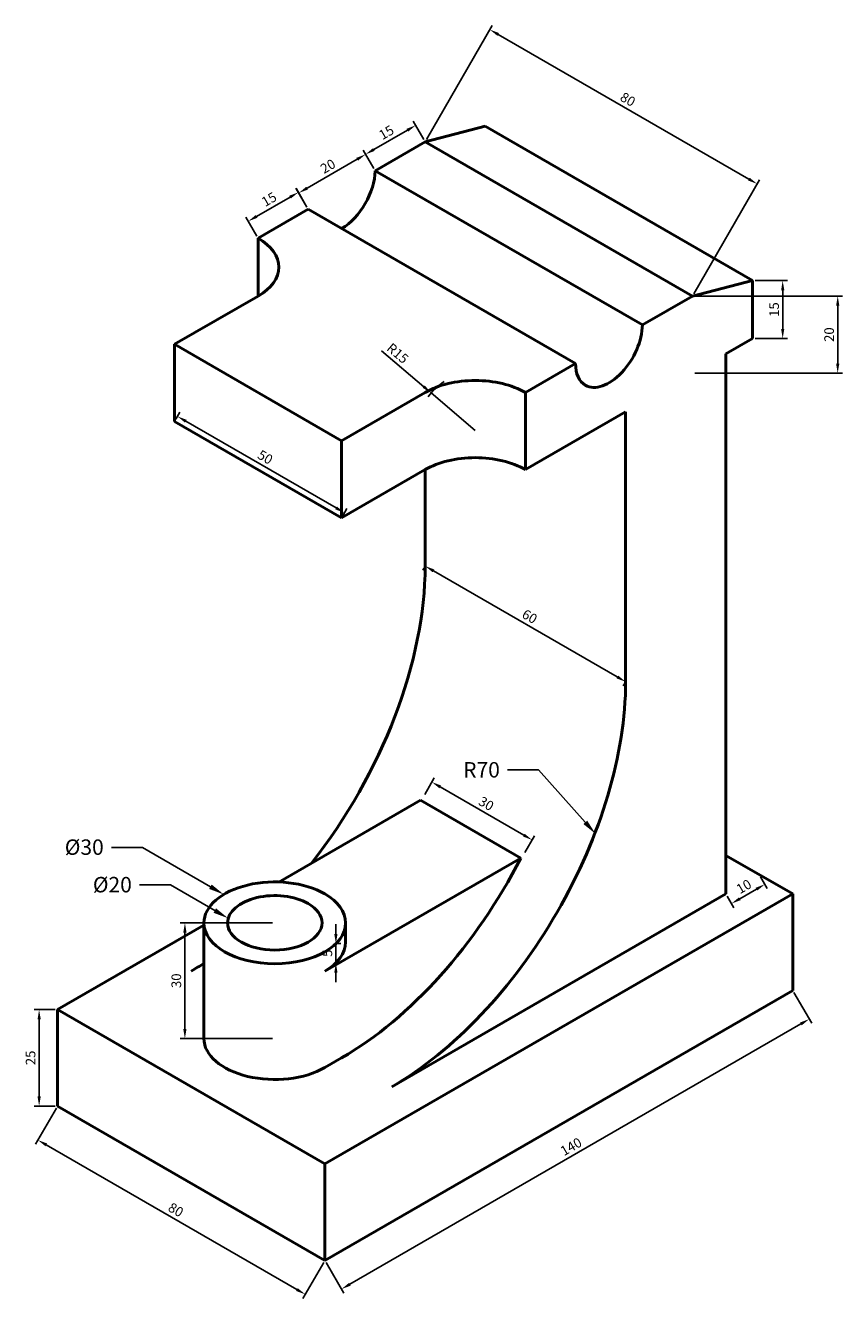
# Model space of a CAD drawing. Units: millimetres. Extents: x 2160 to 2371, y 1190 to 1520.
import ezdxf
from ezdxf import colors
from ezdxf.entities.mleader import LeaderData, LeaderLine
from ezdxf.math import Vec2, Vec3

# ---------------------------------------------------------------- set-up
doc = ezdxf.new("R2010")
doc.units = ezdxf.units.MM
for name, color, linetype, lineweight in [('M-DIMS', 2, 'Continuous', 25), ('M-OUTL', 7, 'Continuous', 50), ('M-TEXT', 3, 'Continuous', 25)]:
    doc.layers.add(name, color=color, linetype=linetype, lineweight=lineweight)
doc.styles.get("Standard").update_dxf_attribs({"font": 'arial.ttf'})
doc.dimstyles.new('ISO-25', dxfattribs={"dimtxt": 2.5, "dimasz": 2.5, "dimexe": 1.25, "dimexo": 0.625, "dimtad": 1, "dimtxsty": 'Standard', "dimcen": 2.5, "dimadec": 0, "dimazin": 0, "dimtfac": 1, "dimtmove": 0, "dimatfit": 3, "dimfxl": 1, "dimarcsym": 0})

# ---------------------------------------------------------------- blocks, each defined once
blk = doc.blocks.new('*D1')
at = {"layer": 'Defpoints', "color": 0, "transparency": 16777216}
for p in [(2167.87, 1239.87), (2237.16, 1199.87), (2232.07, 1191.06)]:
    blk.add_point(p, dxfattribs=at)
at = {"layer": 'M-DIMS', "color": 0, "lineweight": -2, "transparency": 16777216}
for p, q in [((2167.56, 1239.33), (2162.16, 1229.98)), ((2164.95, 1229.81), (2229.9, 1192.31)), ((2236.84, 1199.33), (2231.44, 1189.98))]:
    blk.add_line(p, q, dxfattribs=at)
at = {"layer": 'M-DIMS', "color": 0, "transparency": 16777216}
for points in [[(2165.16, 1230.17), (2164.74, 1229.45), (2162.79, 1231.06)], [(2230.11, 1192.67), (2229.69, 1191.95), (2232.07, 1191.06)]]:
    blk.add_solid(points, dxfattribs=at)
at = {"layer": 'M-DIMS', "color": 0, "transparency": 16777216, "insert": (2198.38, 1212.71), "char_height": 2.5, "attachment_point": 5, "rotation": 330}
blk.add_mtext('80', dxfattribs=at)
blk = doc.blocks.new('*D2')
at = {"layer": 'Defpoints', "color": 0, "transparency": 16777216}
for p in [(2358.4, 1269.87), (2362.7, 1262.43), (2237.16, 1199.87)]:
    blk.add_point(p, dxfattribs=at)
at = {"layer": 'M-DIMS', "color": 0, "lineweight": -2, "transparency": 16777216}
for p, q in [((2358.71, 1269.33), (2363.32, 1261.35)), ((2243.62, 1193.68), (2360.53, 1261.18)), ((2237.47, 1199.33), (2242.08, 1191.35))]:
    blk.add_line(p, q, dxfattribs=at)
at = {"layer": 'M-DIMS', "color": 0, "transparency": 16777216}
for points in [[(2360.32, 1261.54), (2360.74, 1260.82), (2362.7, 1262.43)], [(2243.41, 1194.04), (2243.83, 1193.32), (2241.45, 1192.43)]]:
    blk.add_solid(points, dxfattribs=at)
at = {"layer": 'M-DIMS', "color": 0, "transparency": 16777216, "insert": (2301.12, 1229.08), "char_height": 2.5, "attachment_point": 5, "rotation": 30}
blk.add_mtext('140', dxfattribs=at)
blk = doc.blocks.new('*D3')
at = {"layer": 'Defpoints', "color": 0, "transparency": 16777216}
for p in [(2224.16, 1287.37), (2200.87, 1257.37), (2224.16, 1257.37)]:
    blk.add_point(p, dxfattribs=at)
at = {"layer": 'M-DIMS', "color": 0, "lineweight": -2, "transparency": 16777216}
for p, q in [((2223.54, 1287.37), (2199.62, 1287.37)), ((2200.87, 1284.87), (2200.87, 1259.87)), ((2223.54, 1257.37), (2199.62, 1257.37))]:
    blk.add_line(p, q, dxfattribs=at)
at = {"layer": 'M-DIMS', "color": 0, "transparency": 16777216}
for points in [[(2200.45, 1284.87), (2201.29, 1284.87), (2200.87, 1287.37)], [(2200.45, 1259.87), (2201.29, 1259.87), (2200.87, 1257.37)]]:
    blk.add_solid(points, dxfattribs=at)
at = {"layer": 'M-DIMS', "color": 0, "transparency": 16777216, "insert": (2198.97, 1272.37), "char_height": 2.5, "attachment_point": 5, "rotation": 90}
blk.add_mtext('30', dxfattribs=at)
blk = doc.blocks.new('*D4')
at = {"layer": 'Defpoints', "color": 0, "transparency": 16777216}
for p in [(2240, 1282), (2240, 1277), (2240, 1277)]:
    blk.add_point(p, dxfattribs=at)
at = {"layer": 'M-DIMS', "color": 0, "lineweight": -2, "transparency": 16777216}
for p, q in [((2240, 1284.5), (2240, 1287)), ((2240, 1282), (2240, 1277)), ((2240.63, 1282), (2241.25, 1282)), ((2240, 1274.5), (2240, 1272)), ((2240.63, 1277), (2241.25, 1277))]:
    blk.add_line(p, q, dxfattribs=at)
at = {"layer": 'M-DIMS', "color": 0, "transparency": 16777216}
for points in [[(2239.59, 1284.5), (2240.42, 1284.5), (2240, 1282)], [(2239.59, 1274.5), (2240.42, 1274.5), (2240, 1277)]]:
    blk.add_solid(points, dxfattribs=at)
at = {"layer": 'M-DIMS', "color": 0, "transparency": 16777216, "insert": (2238.11, 1279.5), "char_height": 2.5, "attachment_point": 5, "rotation": 90}
blk.add_mtext('5', dxfattribs=at)
blk = doc.blocks.new('*D5')
at = {"layer": 'Defpoints', "color": 0, "transparency": 16777216}
for p in [(2167.87, 1264.87), (2163.09, 1239.87), (2167.87, 1239.87)]:
    blk.add_point(p, dxfattribs=at)
at = {"layer": 'M-DIMS', "color": 0, "lineweight": -2, "transparency": 16777216}
for p, q in [((2167.25, 1264.87), (2161.84, 1264.87)), ((2163.09, 1262.37), (2163.09, 1242.37)), ((2167.25, 1239.87), (2161.84, 1239.87))]:
    blk.add_line(p, q, dxfattribs=at)
at = {"layer": 'M-DIMS', "color": 0, "transparency": 16777216}
for points in [[(2162.68, 1262.37), (2163.51, 1262.37), (2163.09, 1264.87)], [(2162.68, 1242.37), (2163.51, 1242.37), (2163.09, 1239.87)]]:
    blk.add_solid(points, dxfattribs=at)
at = {"layer": 'M-DIMS', "color": 0, "transparency": 16777216, "insert": (2161.19, 1252.37), "char_height": 2.5, "attachment_point": 5, "rotation": 90}
blk.add_mtext('25', dxfattribs=at)
blk = doc.blocks.new('*D6')
at = {"layer": 'Defpoints', "color": 0, "transparency": 16777216}
for p in [(2262.71, 1320.11), (2290.86, 1308.87), (2288.69, 1305.11)]:
    blk.add_point(p, dxfattribs=at)
at = {"layer": 'M-DIMS', "color": 0, "lineweight": -2, "transparency": 16777216}
for p, q in [((2263.03, 1320.65), (2265.51, 1324.95)), ((2267.05, 1322.62), (2288.7, 1310.12)), ((2289.01, 1305.65), (2291.49, 1309.95))]:
    blk.add_line(p, q, dxfattribs=at)
at = {"layer": 'M-DIMS', "color": 0, "transparency": 16777216}
for points in [[(2267.26, 1322.98), (2266.84, 1322.26), (2264.88, 1323.87)], [(2288.91, 1310.48), (2288.49, 1309.76), (2290.86, 1308.87)]]:
    blk.add_solid(points, dxfattribs=at)
at = {"layer": 'M-DIMS', "color": 0, "transparency": 16777216, "insert": (2278.82, 1318.02), "char_height": 2.5, "attachment_point": 5, "rotation": 330}
blk.add_mtext('30', dxfattribs=at)
blk = doc.blocks.new('*D7')
at = {"layer": 'Defpoints', "color": 0, "transparency": 16777216}
for p in [(2263.14, 1379.87), (2315.1, 1349.87), (2315.1, 1349.87)]:
    blk.add_point(p, dxfattribs=at)
at = {"layer": 'M-DIMS', "color": 0, "lineweight": -2, "transparency": 16777216}
for p, q in [((2262.82, 1379.33), (2262.51, 1378.79)), ((2265.3, 1378.62), (2312.93, 1351.12)), ((2314.78, 1349.33), (2314.47, 1348.79))]:
    blk.add_line(p, q, dxfattribs=at)
at = {"layer": 'M-DIMS', "color": 0, "transparency": 16777216}
for points in [[(2265.51, 1378.99), (2265.09, 1378.26), (2263.14, 1379.87)], [(2313.14, 1351.49), (2312.72, 1350.76), (2315.1, 1349.87)]]:
    blk.add_solid(points, dxfattribs=at)
at = {"layer": 'M-DIMS', "color": 0, "transparency": 16777216, "insert": (2290.07, 1366.52), "char_height": 2.5, "attachment_point": 5, "rotation": 330}
blk.add_mtext('60', dxfattribs=at)
blk = doc.blocks.new('*D8')
at = {"layer": 'Defpoints', "color": 0, "transparency": 16777216}
for p in [(2279.92, 1518.94), (2263.14, 1489.87), (2332.42, 1449.87)]:
    blk.add_point(p, dxfattribs=at)
at = {"layer": 'M-DIMS', "color": 0, "lineweight": -2, "transparency": 16777216}
for p, q in [((2263.45, 1490.42), (2280.54, 1520.02)), ((2347.03, 1480.19), (2282.08, 1517.69)), ((2332.73, 1450.42), (2349.82, 1480.02))]:
    blk.add_line(p, q, dxfattribs=at)
at = {"layer": 'M-DIMS', "color": 0, "transparency": 16777216}
for points in [[(2282.29, 1518.05), (2281.87, 1517.33), (2279.92, 1518.94)], [(2347.24, 1480.55), (2346.83, 1479.83), (2349.2, 1478.94)]]:
    blk.add_solid(points, dxfattribs=at)
at = {"layer": 'M-DIMS', "color": 0, "transparency": 16777216, "insert": (2315.51, 1500.59), "char_height": 2.5, "attachment_point": 5, "rotation": 330}
blk.add_mtext('80', dxfattribs=at)
blk = doc.blocks.new('*D9')
at = {"layer": 'Defpoints', "color": 0, "transparency": 16777216}
for p in [(2348.01, 1453.87), (2348.01, 1438.87), (2355.8, 1438.87)]:
    blk.add_point(p, dxfattribs=at)
at = {"layer": 'M-DIMS', "color": 0, "lineweight": -2, "transparency": 16777216}
for p, q in [((2348.63, 1453.87), (2357.05, 1453.87)), ((2355.8, 1451.37), (2355.8, 1441.37)), ((2348.63, 1438.87), (2357.05, 1438.87))]:
    blk.add_line(p, q, dxfattribs=at)
at = {"layer": 'M-DIMS', "color": 0, "transparency": 16777216}
for points in [[(2355.39, 1451.37), (2356.22, 1451.37), (2355.8, 1453.87)], [(2355.39, 1441.37), (2356.22, 1441.37), (2355.8, 1438.87)]]:
    blk.add_solid(points, dxfattribs=at)
at = {"layer": 'M-DIMS', "color": 0, "transparency": 16777216, "insert": (2353.9, 1446.37), "char_height": 2.5, "attachment_point": 5, "rotation": 90}
blk.add_mtext('15', dxfattribs=at)
blk = doc.blocks.new('*D10')
at = {"layer": 'Defpoints', "color": 0, "transparency": 16777216}
for p in [(2263.14, 1489.87), (2247.7, 1486.62), (2250.15, 1482.37)]:
    blk.add_point(p, dxfattribs=at)
at = {"layer": 'M-DIMS', "color": 0, "lineweight": -2, "transparency": 16777216}
for p, q in [((2262.82, 1490.42), (2260.06, 1495.2)), ((2258.52, 1492.87), (2249.86, 1487.87)), ((2249.83, 1482.92), (2247.07, 1487.7))]:
    blk.add_line(p, q, dxfattribs=at)
at = {"layer": 'M-DIMS', "color": 0, "transparency": 16777216}
for points in [[(2258.31, 1493.23), (2258.73, 1492.5), (2260.69, 1494.12)], [(2249.65, 1488.23), (2250.07, 1487.5), (2247.7, 1486.62)]]:
    blk.add_solid(points, dxfattribs=at)
at = {"layer": 'M-DIMS', "color": 0, "transparency": 16777216, "insert": (2253.24, 1492.01), "char_height": 2.5, "attachment_point": 5, "rotation": 30}
blk.add_mtext('15', dxfattribs=at)
blk = doc.blocks.new('*D11')
at = {"layer": 'Defpoints', "color": 0, "transparency": 16777216}
for p in [(2230.29, 1476.77), (2232.83, 1472.37), (2219.83, 1464.87)]:
    blk.add_point(p, dxfattribs=at)
at = {"layer": 'M-DIMS', "color": 0, "lineweight": -2, "transparency": 16777216}
for p, q in [((2219.46, 1470.52), (2228.12, 1475.52)), ((2232.51, 1472.92), (2229.66, 1477.86)), ((2219.52, 1465.42), (2216.67, 1470.36))]:
    blk.add_line(p, q, dxfattribs=at)
at = {"layer": 'M-DIMS', "color": 0, "transparency": 16777216}
for points in [[(2227.91, 1475.88), (2228.33, 1475.16), (2230.29, 1476.77)], [(2219.25, 1470.88), (2219.67, 1470.16), (2217.3, 1469.27)]]:
    blk.add_solid(points, dxfattribs=at)
at = {"layer": 'M-DIMS', "color": 0, "transparency": 16777216, "insert": (2222.84, 1474.67), "char_height": 2.5, "attachment_point": 5, "rotation": 30}
blk.add_mtext('15', dxfattribs=at)
blk = doc.blocks.new('*D12')
at = {"layer": 'Defpoints', "color": 0, "transparency": 16777216}
for p in [(2247.71, 1486.6), (2250.15, 1482.37), (2232.83, 1472.37)]:
    blk.add_point(p, dxfattribs=at)
at = {"layer": 'M-DIMS', "color": 0, "lineweight": -2, "transparency": 16777216}
for p, q in [((2232.55, 1477.85), (2245.54, 1485.35)), ((2249.83, 1482.92), (2247.08, 1487.68)), ((2232.51, 1472.92), (2229.76, 1477.68))]:
    blk.add_line(p, q, dxfattribs=at)
at = {"layer": 'M-DIMS', "color": 0, "transparency": 16777216}
for points in [[(2245.33, 1485.71), (2245.75, 1484.99), (2247.71, 1486.6)], [(2232.34, 1478.21), (2232.76, 1477.49), (2230.39, 1476.6)]]:
    blk.add_solid(points, dxfattribs=at)
at = {"layer": 'M-DIMS', "color": 0, "transparency": 16777216, "insert": (2238.1, 1483.25), "char_height": 2.5, "attachment_point": 5, "rotation": 30}
blk.add_mtext('20', dxfattribs=at)
blk = doc.blocks.new('*D13')
at = {"layer": 'Defpoints', "color": 0, "transparency": 16777216}
for p in [(2198.18, 1417.37), (2198.94, 1418.68), (2241.49, 1392.37)]:
    blk.add_point(p, dxfattribs=at)
at = {"layer": 'M-DIMS', "color": 0, "lineweight": -2, "transparency": 16777216}
for p, q in [((2198.5, 1417.92), (2199.56, 1419.76)), ((2240.07, 1394.93), (2201.1, 1417.43)), ((2241.8, 1392.92), (2242.86, 1394.76))]:
    blk.add_line(p, q, dxfattribs=at)
at = {"layer": 'M-DIMS', "color": 0, "transparency": 16777216}
for points in [[(2201.31, 1417.79), (2200.89, 1417.07), (2198.94, 1418.68)], [(2240.28, 1395.29), (2239.87, 1394.57), (2242.24, 1393.68)]]:
    blk.add_solid(points, dxfattribs=at)
at = {"layer": 'M-DIMS', "color": 0, "transparency": 16777216, "insert": (2221.54, 1407.83), "char_height": 2.5, "attachment_point": 5, "rotation": 330}
blk.add_mtext('50', dxfattribs=at)
blk = doc.blocks.new('*D14')
at = {"layer": 'Defpoints', "color": 0, "transparency": 16777216}
for p in [(2332.42, 1449.87), (2332.42, 1429.87), (2370.06, 1429.87)]:
    blk.add_point(p, dxfattribs=at)
at = {"layer": 'M-DIMS', "color": 0, "lineweight": -2, "transparency": 16777216}
for p, q in [((2333.04, 1449.87), (2371.31, 1449.87)), ((2370.06, 1447.37), (2370.06, 1432.37)), ((2333.04, 1429.87), (2371.31, 1429.87))]:
    blk.add_line(p, q, dxfattribs=at)
at = {"layer": 'M-DIMS', "color": 0, "transparency": 16777216}
for points in [[(2369.64, 1447.37), (2370.48, 1447.37), (2370.06, 1449.87)], [(2369.64, 1432.37), (2370.48, 1432.37), (2370.06, 1429.87)]]:
    blk.add_solid(points, dxfattribs=at)
at = {"layer": 'M-DIMS', "color": 0, "transparency": 16777216, "insert": (2368.16, 1439.87), "char_height": 2.5, "attachment_point": 5, "rotation": 90}
blk.add_mtext('20', dxfattribs=at)
blk = doc.blocks.new('*D15')
at = {"layer": 'Defpoints', "color": 0, "transparency": 16777216}
for p in [(2349.74, 1299.87), (2351.18, 1297.37), (2341.08, 1294.87)]:
    blk.add_point(p, dxfattribs=at)
at = {"layer": 'M-DIMS', "color": 0, "lineweight": -2, "transparency": 16777216}
for p, q in [((2350.05, 1299.33), (2351.81, 1296.29)), ((2341.39, 1294.33), (2343.15, 1291.29)), ((2344.69, 1293.62), (2349.02, 1296.12))]:
    blk.add_line(p, q, dxfattribs=at)
at = {"layer": 'M-DIMS', "color": 0, "transparency": 16777216}
for points in [[(2348.81, 1296.48), (2349.23, 1295.76), (2351.18, 1297.37)], [(2344.48, 1293.98), (2344.9, 1293.26), (2342.52, 1292.37)]]:
    blk.add_solid(points, dxfattribs=at)
at = {"layer": 'M-DIMS', "color": 0, "transparency": 16777216, "insert": (2345.9, 1296.52), "char_height": 2.5, "attachment_point": 5, "rotation": 30}
blk.add_mtext('10', dxfattribs=at)
blk = doc.blocks.new('*D16')
at = {"layer": 'Defpoints', "color": 0, "transparency": 16777216}
for p in [(2264.69, 1424.76), (2276.13, 1415.05)]:
    blk.add_point(p, dxfattribs=at)
at = {"layer": 'M-DIMS', "color": 0, "lineweight": -2, "transparency": 16777216}
for p, q in [((2251.82, 1435.68), (2262.78, 1426.38)), ((2276.13, 1415.05), (2264.69, 1424.76))]:
    blk.add_line(p, q, dxfattribs=at)
blk.add_arc((2276.13, 1415.05), 15, 122.3873, 144.4624, dxfattribs=at)
at = {"layer": 'M-DIMS', "color": 0, "transparency": 16777216}
blk.add_solid([(2263.05, 1426.69), (2262.51, 1426.06), (2264.69, 1424.76)], dxfattribs=at)
at = {"layer": 'M-DIMS', "color": 0, "transparency": 16777216, "insert": (2255.81, 1434.79), "char_height": 2.5, "attachment_point": 5, "rotation": 319.6878}
blk.add_mtext('R15', dxfattribs=at)

msp = doc.modelspace()

# ---------------------------------------------------------------- linework, layer by layer
at = {"layer": 'M-OUTL'}
for p, q in [((2278.724, 1493.874), (2263.136, 1489.874)), ((2348.006, 1453.874), (2278.724, 1493.874)), ((2263.136, 1489.874), (2250.146, 1482.374)), ((2332.418, 1449.874), (2263.136, 1489.874)), ((2319.428, 1442.374), (2250.146, 1482.374)), ((2232.825, 1472.374), (2219.835, 1464.874)), ((2302.107, 1432.374), (2232.825, 1472.374)), ((2219.835, 1464.874), (2219.835, 1449.874)), ((2348.006, 1453.874), (2332.418, 1449.874)), ((2348.006, 1438.874), (2348.006, 1453.874)), ((2219.835, 1449.874), (2198.184, 1437.374)), ((2332.418, 1449.874), (2319.428, 1442.374)), ((2198.184, 1417.374), (2198.184, 1437.374)), ((2198.184, 1437.374), (2241.485, 1412.374)), ((2341.078, 1434.874), (2348.006, 1438.874)), ((2341.078, 1434.874), (2341.078, 1294.874)), ((2302.107, 1432.374), (2289.117, 1424.874)), ((2241.485, 1412.374), (2263.136, 1424.874)), ((2289.117, 1424.874), (2289.117, 1404.874)), ((2289.117, 1404.874), (2315.098, 1419.874)), ((2315.098, 1349.874), (2315.098, 1419.874)), ((2198.184, 1417.374), (2241.485, 1392.374)), ((2241.485, 1392.374), (2241.485, 1412.374)), ((2241.485, 1392.374), (2263.136, 1404.874)), ((2263.136, 1379.874), (2263.136, 1404.874)), ((2225.187, 1297.965), (2261.94, 1319.184)), ((2261.94, 1319.184), (2287.921, 1304.184)), ((2237.155, 1274.874), (2287.921, 1304.184)), ((2358.399, 1294.874), (2341.078, 1304.874)), ((2237.155, 1224.874), (2358.399, 1294.874)), ((2341.078, 1294.874), (2254.476, 1244.874)), ((2358.399, 1269.874), (2358.399, 1294.874)), ((2205.794, 1257.374), (2205.794, 1287.374)), ((2242.536, 1282.374), (2242.536, 1287.374)), ((2167.873, 1264.874), (2205.794, 1286.768)), ((2237.155, 1199.874), (2358.399, 1269.874)), ((2237.155, 1224.874), (2167.873, 1264.874)), ((2167.873, 1239.874), (2167.873, 1264.874)), ((2237.155, 1249.874), (2241.485, 1252.374)), ((2237.155, 1199.874), (2167.873, 1239.874)), ((2237.155, 1199.874), (2237.155, 1224.874))]:
    msp.add_line(p, q, dxfattribs=at)
for centre, major_axis, start_param, end_param in [((2241.485, 1477.374), (6.124, 10.607), 3.9269908, 5.4977871), ((2206.844, 1457.374), (-18.371, 0), 3.1415927, 3.9269909), ((2206.844, 1457.374), (-18.371, 0), 2.3561944, 3.1415927), ((2310.767, 1437.374), (6.124, 10.607), 3.1415927, 5.4977871), ((2310.767, 1437.374), (6.124, 10.607), 2.3561945, 3.1415927), ((2276.126, 1417.374), (-18.371, 0), 3.9269908, 5.4977872), ((2276.126, 1397.374), (-18.371, 0), 3.9269908, 5.4977872), ((2202.514, 1344.874), (-42.866, -74.246), 1.3264977, 2.3561945), ((2254.476, 1314.874), (-42.866, -74.246), 0.7853981, 2.3561945), ((2241.485, 1322.374), (-42.866, -74.246), 0.7853981, 1.657972), ((2224.165, 1287.374), (18.371, 0), 0.7853982, 3.1415927), ((2224.165, 1287.374), (12.247, 0), 0.7853982, 3.1415927), ((2224.165, 1287.374), (18.371, 0), 0, 0.7853982), ((2224.165, 1287.374), (12.247, 0), 0, 0.7853982), ((2224.165, 1287.374), (18.371, 0), 3.1415927, 6.2831853), ((2224.165, 1287.374), (12.247, 0), 3.1415927, 6.2831853), ((2224.165, 1282.374), (18.371, 0), 5.4977871, 6.2831853), ((2202.514, 1344.874), (-42.866, -74.246), 0.7853981, 0.8395217), ((2224.165, 1257.374), (18.371, 0), 3.1415927, 5.4977871)]:
    msp.add_ellipse(centre, major_axis=major_axis, ratio=0.5773503, start_param=start_param, end_param=end_param, dxfattribs=at)

# ---------------------------------------------------------------- dimensions: what is measured, and where the dimension line sits
at = {"layer": 'M-DIMS'}
for p1, p2, distance, picture, middle in [((2332.418, 1449.874), (2263.136, 1489.874), -33.562, '*D8', (2315.509, 1500.586)), ((2263.136, 1489.874), (2250.146, 1482.374), -4.897, '*D10', (2253.242, 1492.012)), ((2232.825, 1472.374), (2250.146, 1482.374), 4.878, '*D12', (2238.095, 1483.246)), ((2219.835, 1464.874), (2232.825, 1472.374), 5.079, '*D11', (2222.84, 1474.67)), ((2348.006, 1453.874), (2348.006, 1438.874), 7.796, '*D9', (2353.901, 1446.374)), ((2241.485, 1392.374), (2198.184, 1417.374), -1.507, '*D13', (2221.539, 1407.827)), ((2263.136, 1379.875), (2315.097, 1349.875), 0, '*D7', (2290.067, 1366.521)), ((2262.713, 1320.111), (2288.694, 1305.111), 4.34, '*D6', (2278.825, 1318.017)), ((2341.078, 1294.874), (2349.739, 1299.874), -2.891, '*D15', (2345.903, 1296.518)), ((2224.165, 1287.374), (2224.165, 1257.374), -23.295, '*D3', (2198.968, 1272.374)), ((2240.002, 1281.999), (2240.002, 1276.999), 0, '*D4', (2238.106, 1279.499)), ((2237.155, 1199.874), (2358.399, 1269.874), -8.594, '*D2', (2301.123, 1229.078)), ((2167.873, 1264.874), (2167.873, 1239.874), -4.781, '*D5', (2161.191, 1252.374)), ((2167.873, 1239.874), (2237.155, 1199.874), -10.175, '*D1', (2198.377, 1212.709))]:
    dim = msp.add_aligned_dim(p1=p1, p2=p2, distance=distance, dimstyle='ISO-25', override={"dimclrd": 0, "dimclre": 0, "dimclrt": 0}, dxfattribs=at)
    dim.commit()
    dim.dimension.update_dxf_attribs({"geometry": picture, "text_midpoint": middle})
dim = msp.add_linear_dim(base=(2370.061, 1429.874), p1=(2332.418, 1449.874), p2=(2332.418, 1429.874), angle=90, dimstyle='ISO-25', override={"dimclrd": 0, "dimclre": 0, "dimclrt": 0}, dxfattribs=at)
dim.commit()
dim.dimension.update_dxf_attribs({"geometry": '*D14', "text_midpoint": (2368.16, 1439.874)})
dim = msp.add_radius_dim(center=(2276.126, 1415.054), mpoint=(2264.688, 1424.758), dimstyle='ISO-25', override={"dimclrd": 0, "dimclre": 0, "dimclrt": 0}, dxfattribs=at)
dim.commit()
dim.dimension.update_dxf_attribs({"geometry": '*D16', "text_midpoint": (2254.579, 1433.335), "dimtype": 164})

# ---------------------------------------------------------------- leaders
at = {"layer": 'M-TEXT'}
ml = msp.add_multileader_mtext('Standard', dxfattribs=at)
ml.set_content('R70', color=256)
ml.set_leader_properties()
ml.build(insert=Vec2(0, 0))
ctx = ml.context
ctx.base_point, ctx.plane_origin = Vec3(2270.955, 1327.019), Vec3(2307.311, 1310.453)
ctx.text_align_type = 2
notes = []
notes.append((ctx, [(0, (1, 1, 0), (2292.5, 1327.019), (-1, 0), 8, [(0, [(2307.311, 1310.453)], 0, [])])]))
ctx.mtext.insert, ctx.mtext.alignment, ctx.mtext.flow_direction = Vec3(2282.5, 1329.053), 3, 5
ml = msp.add_multileader_mtext('Standard', dxfattribs=at)
ml.set_content('%%C30', color=256)
ml.set_leader_properties()
ml.build(insert=Vec2(0, 0))
ctx = ml.context
ctx.base_point, ctx.plane_origin = Vec3(2167.772, 1306.924), Vec3(2210.945, 1294.739)
ctx.text_align_type = 2
notes.append((ctx, [(0, (1, 1, 0), (2189.84, 1306.924), (-1, 0), 8, [(0, [(2210.945, 1294.739)], 0, [])])]))
ctx.mtext.insert, ctx.mtext.alignment, ctx.mtext.flow_direction = Vec3(2179.84, 1309.005), 3, 5
ml = msp.add_multileader_mtext('Standard', dxfattribs=at)
ml.set_content('%%C20', color=256)
ml.set_leader_properties()
ml.build(insert=Vec2(0, 0))
ctx = ml.context
ctx.base_point, ctx.plane_origin = Vec3(2175.052, 1297.198), Vec3(2212.089, 1288.556)
ctx.text_align_type = 2
notes.append((ctx, [(0, (1, 1, 0), (2197.12, 1297.198), (-1, 0), 8, [(0, [(2212.089, 1288.556)], 0, [])])]))
ctx.mtext.insert, ctx.mtext.alignment, ctx.mtext.flow_direction = Vec3(2187.12, 1299.279), 3, 5
for ctx, leaders in notes:
    for number, flags, end, landing, length, lines in leaders:
        leader = LeaderData()
        leader.index, (leader.has_last_leader_line, leader.has_dogleg_vector, leader.attachment_direction) = number, flags
        leader.last_leader_point, leader.dogleg_vector, leader.dogleg_length = Vec3(end), Vec3(landing), length
        for number, points, colour, breaks in lines:
            line = LeaderLine()
            line.index, line.vertices, line.color, line.breaks = number, Vec3.list(points), colors.encode_raw_color(colour), breaks
            leader.lines.append(line)
        ctx.leaders.append(leader)

doc.saveas('drawing.dxf')
